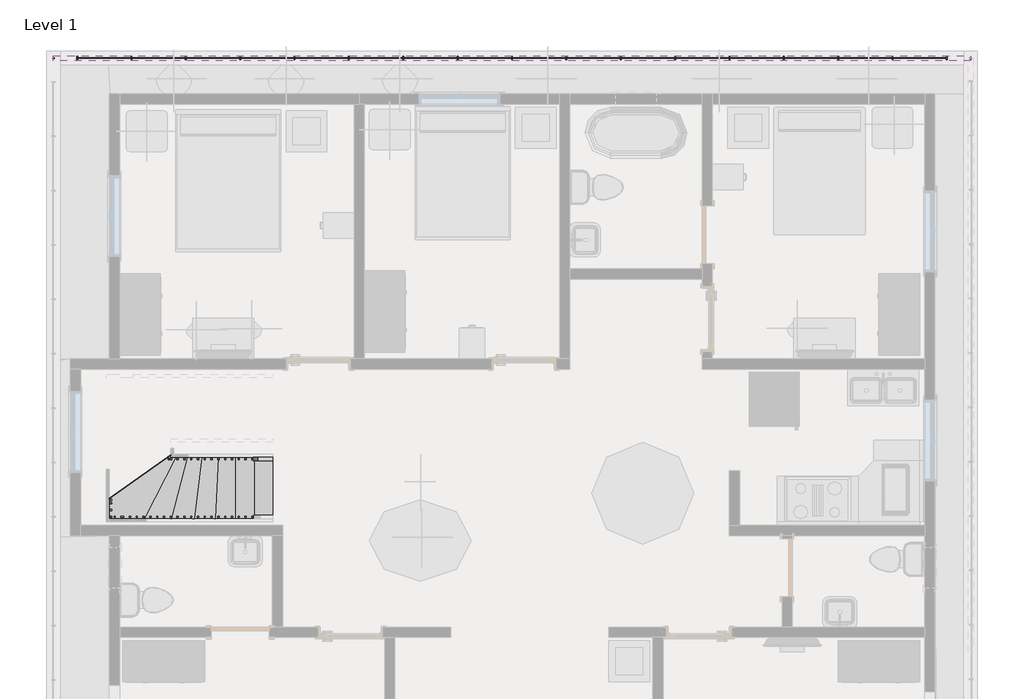
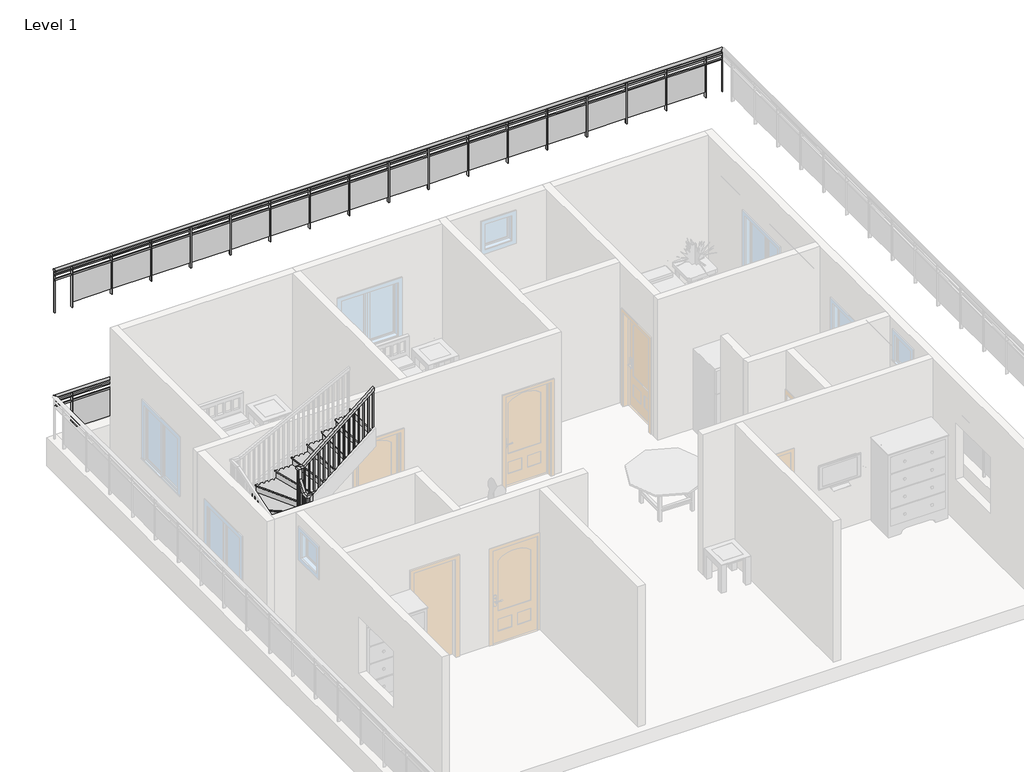
# One storey, part 3 of 5: 3 railings, 1 stair flight.
"""IFC4 building model written with IfcOpenShell, lengths in millimetres."""

from ifc_helpers import new_model, si_unit, point, frame, origin, place, context, project, spatial, polyline, ellipse_curve, trimmed, outline, extrude, faceted_brep, transform, mapped, element, save
from ifc_brep_helpers import plane_surface, extruded_surface, advanced_brep
from components import stair_flight_b82eb699

model = new_model("IFC4")

# Units and contexts
model_context = context("Model", 3, world=origin())
ifc_project = project(units=[si_unit("LENGTHUNIT", "METRE", prefix="MILLI")], contexts=[model_context])

# Site, building, storey
site = spatial("IfcSite", under=ifc_project)
building = spatial("IfcBuilding", under=site)
storey = spatial("IfcBuildingStorey", under=building, Name="Level 1", Elevation=0.0)

# Railings
placement = place(None, origin())
element("IfcRailing", 1, ObjectType="Glass Panel - Bottom Fill", at=placement, inside=storey, context=model_context, shape_type="SolidModel", body=[
    advanced_brep(
    [(-11479.0434666, 14380.2716937, 4267.2), (-11479.0434666, 14304.0716937, 4267.2), (2236.9565334, 14380.2716937, 4267.2), (2236.9565334, 14304.0716937, 4267.2)],
    [
        (0, 1, ellipse_curve(frame((-11479.0434666, 14342.1716937, 4267.2), z_axis=(-1.0, 0.0, 0.0), x_axis=(0.0, -1.0, 0.0)), 38.1, 28.575)),
        (1, 0, ellipse_curve(frame((-11479.0434666, 14342.1716937, 4267.2), z_axis=(-1.0, 0.0, 0.0), x_axis=(0.0, -1.0, 0.0)), 38.1, 28.575)),
        (2, 3, ellipse_curve(frame((2236.9565334, 14342.1716937, 4267.2), z_axis=(1.0, 0.0, 0.0), x_axis=(0.0, -1.0, 0.0)), 38.1, 28.575)),
        (3, 2, ellipse_curve(frame((2236.9565334, 14342.1716937, 4267.2), z_axis=(1.0, 0.0, 0.0), x_axis=(0.0, -1.0, 0.0)), 38.1, 28.575)),
        (0, 2),
        (3, 1),
    ],
    [
        plane_surface(frame((-11479.0434666, 14342.1716937, 4267.2), z_axis=(-1.0, 0.0, 0.0), x_axis=(0.0, 1.0, 0.0))),
        plane_surface(frame((2236.9565334, 14342.1716937, 4267.2), z_axis=(1.0, 0.0, 0.0), x_axis=(0.0, 1.0, 0.0))),
        extruded_surface(trimmed(ellipse_curve(frame((2236.9565334, 14342.1716937, 4267.2), z_axis=(-1.0, 0.0, 0.0), x_axis=(0.0, -1.0, 0.0)), 38.1, 28.575), [point((2236.9565334, 14380.2716937, 4267.2))], [point((2236.9565334, 14304.0716937, 4267.2))], True, "CARTESIAN"), (-13716.0, 0.0, 0.0), 13716.0),
        extruded_surface(trimmed(ellipse_curve(frame((2236.9565334, 14342.1716937, 4267.2), z_axis=(-1.0, 0.0, 0.0), x_axis=(0.0, -1.0, 0.0)), 38.1, 28.575), [point((2236.9565334, 14304.0716937, 4267.2))], [point((2236.9565334, 14380.2716937, 4267.2))], True, "CARTESIAN"), (-13716.0, 0.0, 0.0), 13716.0),
    ],
    [
        (0, [[1, 2]]),
        (1, [[3, 4]]),
        (2, [[-1, 5, -4, 6]]),
        (3, [[-2, -6, -3, -5]]),
    ],
),
    extrude(outline(polyline([(-11479.0434666, 14329.4716937), (-11479.0434666, 14354.8716937), (2236.9565334, 14354.8716937), (2236.9565334, 14329.4716937), (-11479.0434666, 14329.4716937)])), frame((0.0, 0.0, 4152.9), z_axis=(0.0, 0.0, 1.0), x_axis=(1.0, 0.0, 0.0)), (0.0, 0.0, 1.0), 25.4),
    extrude(outline(polyline([(-11479.0434666, 14329.4716937), (-11479.0434666, 14354.8716937), (2236.9565334, 14354.8716937), (2236.9565334, 14329.4716937), (-11479.0434666, 14329.4716937)])), frame((0.0, 0.0, 4051.3), z_axis=(0.0, 0.0, 1.0), x_axis=(1.0, 0.0, 0.0)), (0.0, 0.0, 1.0), 25.4),
    extrude(outline(polyline([(1875.0065334, 14316.7716937), (1875.0065334, 14367.5716937), (1887.7065334, 14367.5716937), (1887.7065334, 14316.7716937), (1875.0065334, 14316.7716937)])), frame((0.0, 0.0, 3352.8), z_axis=(0.0, 0.0, 1.0), x_axis=(1.0, 0.0, 0.0)), (0.0, 0.0, 1.0), 885.6788223),
    extrude(outline(polyline([(1068.5565334, 14348.7068507), (1881.3565334, 14348.7068507), (1881.3565334, 14342.3568507), (1068.5565334, 14342.3568507), (1068.5565334, 14348.7068507)])), frame((0.0, 0.0, 3454.4), z_axis=(0.0, 0.0, 1.0), x_axis=(1.0, 0.0, 0.0)), (0.0, 0.0, 1.0), 596.9),
    extrude(outline(polyline([(1062.2065334, 14316.7716937), (1062.2065334, 14367.5716937), (1074.9065334, 14367.5716937), (1074.9065334, 14316.7716937), (1062.2065334, 14316.7716937)])), frame((0.0, 0.0, 3352.8), z_axis=(0.0, 0.0, 1.0), x_axis=(1.0, 0.0, 0.0)), (0.0, 0.0, 1.0), 885.6788223),
    extrude(outline(polyline([(255.7565334, 14348.7068507), (1068.5565334, 14348.7068507), (1068.5565334, 14342.3568507), (255.7565334, 14342.3568507), (255.7565334, 14348.7068507)])), frame((0.0, 0.0, 3454.4), z_axis=(0.0, 0.0, 1.0), x_axis=(1.0, 0.0, 0.0)), (0.0, 0.0, 1.0), 596.9),
    extrude(outline(polyline([(249.4065334, 14316.7716937), (249.4065334, 14367.5716937), (262.1065334, 14367.5716937), (262.1065334, 14316.7716937), (249.4065334, 14316.7716937)])), frame((0.0, 0.0, 3352.8), z_axis=(0.0, 0.0, 1.0), x_axis=(1.0, 0.0, 0.0)), (0.0, 0.0, 1.0), 885.6788223),
    extrude(outline(polyline([(-557.0434666, 14348.7068507), (255.7565334, 14348.7068507), (255.7565334, 14342.3568507), (-557.0434666, 14342.3568507), (-557.0434666, 14348.7068507)])), frame((0.0, 0.0, 3454.4), z_axis=(0.0, 0.0, 1.0), x_axis=(1.0, 0.0, 0.0)), (0.0, 0.0, 1.0), 596.9),
    extrude(outline(polyline([(-563.3934666, 14316.7716937), (-563.3934666, 14367.5716937), (-550.6934666, 14367.5716937), (-550.6934666, 14316.7716937), (-563.3934666, 14316.7716937)])), frame((0.0, 0.0, 3352.8), z_axis=(0.0, 0.0, 1.0), x_axis=(1.0, 0.0, 0.0)), (0.0, 0.0, 1.0), 885.6788223),
    extrude(outline(polyline([(-1369.8434666, 14348.7068507), (-557.0434666, 14348.7068507), (-557.0434666, 14342.3568507), (-1369.8434666, 14342.3568507), (-1369.8434666, 14348.7068507)])), frame((0.0, 0.0, 3454.4), z_axis=(0.0, 0.0, 1.0), x_axis=(1.0, 0.0, 0.0)), (0.0, 0.0, 1.0), 596.9),
    extrude(outline(polyline([(-1376.1934666, 14316.7716937), (-1376.1934666, 14367.5716937), (-1363.4934666, 14367.5716937), (-1363.4934666, 14316.7716937), (-1376.1934666, 14316.7716937)])), frame((0.0, 0.0, 3352.8), z_axis=(0.0, 0.0, 1.0), x_axis=(1.0, 0.0, 0.0)), (0.0, 0.0, 1.0), 885.6788223),
    extrude(outline(polyline([(-2182.6434666, 14348.7068507), (-1369.8434666, 14348.7068507), (-1369.8434666, 14342.3568507), (-2182.6434666, 14342.3568507), (-2182.6434666, 14348.7068507)])), frame((0.0, 0.0, 3454.4), z_axis=(0.0, 0.0, 1.0), x_axis=(1.0, 0.0, 0.0)), (0.0, 0.0, 1.0), 596.9),
    extrude(outline(polyline([(-2188.9934666, 14316.7716937), (-2188.9934666, 14367.5716937), (-2176.2934666, 14367.5716937), (-2176.2934666, 14316.7716937), (-2188.9934666, 14316.7716937)])), frame((0.0, 0.0, 3352.8), z_axis=(0.0, 0.0, 1.0), x_axis=(1.0, 0.0, 0.0)), (0.0, 0.0, 1.0), 885.6788223),
    extrude(outline(polyline([(-2995.4434666, 14348.7068507), (-2182.6434666, 14348.7068507), (-2182.6434666, 14342.3568507), (-2995.4434666, 14342.3568507), (-2995.4434666, 14348.7068507)])), frame((0.0, 0.0, 3454.4), z_axis=(0.0, 0.0, 1.0), x_axis=(1.0, 0.0, 0.0)), (0.0, 0.0, 1.0), 596.9),
    extrude(outline(polyline([(-3001.7934666, 14316.7716937), (-3001.7934666, 14367.5716937), (-2989.0934666, 14367.5716937), (-2989.0934666, 14316.7716937), (-3001.7934666, 14316.7716937)])), frame((0.0, 0.0, 3352.8), z_axis=(0.0, 0.0, 1.0), x_axis=(1.0, 0.0, 0.0)), (0.0, 0.0, 1.0), 885.6788223),
    extrude(outline(polyline([(-3808.2434666, 14348.7068507), (-2995.4434666, 14348.7068507), (-2995.4434666, 14342.3568507), (-3808.2434666, 14342.3568507), (-3808.2434666, 14348.7068507)])), frame((0.0, 0.0, 3454.4), z_axis=(0.0, 0.0, 1.0), x_axis=(1.0, 0.0, 0.0)), (0.0, 0.0, 1.0), 596.9),
    extrude(outline(polyline([(-3814.5934666, 14316.7716937), (-3814.5934666, 14367.5716937), (-3801.8934666, 14367.5716937), (-3801.8934666, 14316.7716937), (-3814.5934666, 14316.7716937)])), frame((0.0, 0.0, 3352.8), z_axis=(0.0, 0.0, 1.0), x_axis=(1.0, 0.0, 0.0)), (0.0, 0.0, 1.0), 885.6788223),
    extrude(outline(polyline([(-4621.0434666, 14348.7068507), (-3808.2434666, 14348.7068507), (-3808.2434666, 14342.3568507), (-4621.0434666, 14342.3568507), (-4621.0434666, 14348.7068507)])), frame((0.0, 0.0, 3454.4), z_axis=(0.0, 0.0, 1.0), x_axis=(1.0, 0.0, 0.0)), (0.0, 0.0, 1.0), 596.9),
    extrude(outline(polyline([(-4627.3934666, 14316.7716937), (-4627.3934666, 14367.5716937), (-4614.6934666, 14367.5716937), (-4614.6934666, 14316.7716937), (-4627.3934666, 14316.7716937)])), frame((0.0, 0.0, 3352.8), z_axis=(0.0, 0.0, 1.0), x_axis=(1.0, 0.0, 0.0)), (0.0, 0.0, 1.0), 885.6788223),
    extrude(outline(polyline([(-5433.8434666, 14348.7068507), (-4621.0434666, 14348.7068507), (-4621.0434666, 14342.3568507), (-5433.8434666, 14342.3568507), (-5433.8434666, 14348.7068507)])), frame((0.0, 0.0, 3454.4), z_axis=(0.0, 0.0, 1.0), x_axis=(1.0, 0.0, 0.0)), (0.0, 0.0, 1.0), 596.9),
    extrude(outline(polyline([(-5440.1934666, 14316.7716937), (-5440.1934666, 14367.5716937), (-5427.4934666, 14367.5716937), (-5427.4934666, 14316.7716937), (-5440.1934666, 14316.7716937)])), frame((0.0, 0.0, 3352.8), z_axis=(0.0, 0.0, 1.0), x_axis=(1.0, 0.0, 0.0)), (0.0, 0.0, 1.0), 885.6788223),
    extrude(outline(polyline([(-6246.6434666, 14348.7068507), (-5433.8434666, 14348.7068507), (-5433.8434666, 14342.3568507), (-6246.6434666, 14342.3568507), (-6246.6434666, 14348.7068507)])), frame((0.0, 0.0, 3454.4), z_axis=(0.0, 0.0, 1.0), x_axis=(1.0, 0.0, 0.0)), (0.0, 0.0, 1.0), 596.9),
    extrude(outline(polyline([(-6252.9934666, 14316.7716937), (-6252.9934666, 14367.5716937), (-6240.2934666, 14367.5716937), (-6240.2934666, 14316.7716937), (-6252.9934666, 14316.7716937)])), frame((0.0, 0.0, 3352.8), z_axis=(0.0, 0.0, 1.0), x_axis=(1.0, 0.0, 0.0)), (0.0, 0.0, 1.0), 885.6788223),
    extrude(outline(polyline([(-7059.4434666, 14348.7068507), (-6246.6434666, 14348.7068507), (-6246.6434666, 14342.3568507), (-7059.4434666, 14342.3568507), (-7059.4434666, 14348.7068507)])), frame((0.0, 0.0, 3454.4), z_axis=(0.0, 0.0, 1.0), x_axis=(1.0, 0.0, 0.0)), (0.0, 0.0, 1.0), 596.9),
    extrude(outline(polyline([(-7065.7934666, 14316.7716937), (-7065.7934666, 14367.5716937), (-7053.0934666, 14367.5716937), (-7053.0934666, 14316.7716937), (-7065.7934666, 14316.7716937)])), frame((0.0, 0.0, 3352.8), z_axis=(0.0, 0.0, 1.0), x_axis=(1.0, 0.0, 0.0)), (0.0, 0.0, 1.0), 885.6788223),
    extrude(outline(polyline([(-7872.2434666, 14348.7068507), (-7059.4434666, 14348.7068507), (-7059.4434666, 14342.3568507), (-7872.2434666, 14342.3568507), (-7872.2434666, 14348.7068507)])), frame((0.0, 0.0, 3454.4), z_axis=(0.0, 0.0, 1.0), x_axis=(1.0, 0.0, 0.0)), (0.0, 0.0, 1.0), 596.9),
    extrude(outline(polyline([(-7878.5934666, 14316.7716937), (-7878.5934666, 14367.5716937), (-7865.8934666, 14367.5716937), (-7865.8934666, 14316.7716937), (-7878.5934666, 14316.7716937)])), frame((0.0, 0.0, 3352.8), z_axis=(0.0, 0.0, 1.0), x_axis=(1.0, 0.0, 0.0)), (0.0, 0.0, 1.0), 885.6788223),
    extrude(outline(polyline([(-8685.0434666, 14348.7068507), (-7872.2434666, 14348.7068507), (-7872.2434666, 14342.3568507), (-8685.0434666, 14342.3568507), (-8685.0434666, 14348.7068507)])), frame((0.0, 0.0, 3454.4), z_axis=(0.0, 0.0, 1.0), x_axis=(1.0, 0.0, 0.0)), (0.0, 0.0, 1.0), 596.9),
    extrude(outline(polyline([(-8691.3934666, 14316.7716937), (-8691.3934666, 14367.5716937), (-8678.6934666, 14367.5716937), (-8678.6934666, 14316.7716937), (-8691.3934666, 14316.7716937)])), frame((0.0, 0.0, 3352.8), z_axis=(0.0, 0.0, 1.0), x_axis=(1.0, 0.0, 0.0)), (0.0, 0.0, 1.0), 885.6788223),
    extrude(outline(polyline([(-9497.8434666, 14348.7068507), (-8685.0434666, 14348.7068507), (-8685.0434666, 14342.3568507), (-9497.8434666, 14342.3568507), (-9497.8434666, 14348.7068507)])), frame((0.0, 0.0, 3454.4), z_axis=(0.0, 0.0, 1.0), x_axis=(1.0, 0.0, 0.0)), (0.0, 0.0, 1.0), 596.9),
    extrude(outline(polyline([(-9504.1934666, 14316.7716937), (-9504.1934666, 14367.5716937), (-9491.4934666, 14367.5716937), (-9491.4934666, 14316.7716937), (-9504.1934666, 14316.7716937)])), frame((0.0, 0.0, 3352.8), z_axis=(0.0, 0.0, 1.0), x_axis=(1.0, 0.0, 0.0)), (0.0, 0.0, 1.0), 885.6788223),
    extrude(outline(polyline([(-10310.6434666, 14348.7068507), (-9497.8434666, 14348.7068507), (-9497.8434666, 14342.3568507), (-10310.6434666, 14342.3568507), (-10310.6434666, 14348.7068507)])), frame((0.0, 0.0, 3454.4), z_axis=(0.0, 0.0, 1.0), x_axis=(1.0, 0.0, 0.0)), (0.0, 0.0, 1.0), 596.9),
    extrude(outline(polyline([(-10316.9934666, 14316.7716937), (-10316.9934666, 14367.5716937), (-10304.2934666, 14367.5716937), (-10304.2934666, 14316.7716937), (-10316.9934666, 14316.7716937)])), frame((0.0, 0.0, 3352.8), z_axis=(0.0, 0.0, 1.0), x_axis=(1.0, 0.0, 0.0)), (0.0, 0.0, 1.0), 885.6788223),
    extrude(outline(polyline([(-11123.4434666, 14348.7068507), (-10310.6434666, 14348.7068507), (-10310.6434666, 14342.3568507), (-11123.4434666, 14342.3568507), (-11123.4434666, 14348.7068507)])), frame((0.0, 0.0, 3454.4), z_axis=(0.0, 0.0, 1.0), x_axis=(1.0, 0.0, 0.0)), (0.0, 0.0, 1.0), 596.9),
    extrude(outline(polyline([(-11129.7934666, 14316.7716937), (-11129.7934666, 14367.5716937), (-11117.0934666, 14367.5716937), (-11117.0934666, 14316.7716937), (-11129.7934666, 14316.7716937)])), frame((0.0, 0.0, 3352.8), z_axis=(0.0, 0.0, 1.0), x_axis=(1.0, 0.0, 0.0)), (0.0, 0.0, 1.0), 885.6788223),
    extrude(outline(polyline([(2224.2565334, 14332.6466937), (2224.2565334, 14351.6966937), (2243.3065334, 14351.6966937), (2243.3065334, 14332.6466937), (2224.2565334, 14332.6466937)])), frame((0.0, 0.0, 3352.8), z_axis=(0.0, 0.0, 1.0), x_axis=(1.0, 0.0, 0.0)), (0.0, 0.0, 1.0), 885.6788223),
    extrude(outline(polyline([(-11485.3934666, 14332.6466937), (-11485.3934666, 14351.6966937), (-11466.3434666, 14351.6966937), (-11466.3434666, 14332.6466937), (-11485.3934666, 14332.6466937)])), frame((0.0, 0.0, 3352.8), z_axis=(0.0, 0.0, 1.0), x_axis=(1.0, 0.0, 0.0)), (0.0, 0.0, 1.0), 885.6788223),
])
element("IfcRailing", 2, ObjectType="Glass Panel - Bottom Fill", at=placement, inside=storey, context=model_context, shape_type="SolidModel", body=[
    advanced_brep(
    [(-11479.0434666, 14380.2716937, 1524.0), (-11479.0434666, 14304.0716937, 1524.0), (2236.9565334, 14380.2716937, 1524.0), (2236.9565334, 14304.0716937, 1524.0)],
    [
        (0, 1, ellipse_curve(frame((-11479.0434666, 14342.1716937, 1524.0), z_axis=(-1.0, 0.0, 0.0), x_axis=(0.0, -1.0, 0.0)), 38.1, 28.575)),
        (1, 0, ellipse_curve(frame((-11479.0434666, 14342.1716937, 1524.0), z_axis=(-1.0, 0.0, 0.0), x_axis=(0.0, -1.0, 0.0)), 38.1, 28.575)),
        (2, 3, ellipse_curve(frame((2236.9565334, 14342.1716937, 1524.0), z_axis=(1.0, 0.0, 0.0), x_axis=(0.0, -1.0, 0.0)), 38.1, 28.575)),
        (3, 2, ellipse_curve(frame((2236.9565334, 14342.1716937, 1524.0), z_axis=(1.0, 0.0, 0.0), x_axis=(0.0, -1.0, 0.0)), 38.1, 28.575)),
        (0, 2),
        (3, 1),
    ],
    [
        plane_surface(frame((-11479.0434666, 14342.1716937, 1524.0), z_axis=(-1.0, 0.0, 0.0), x_axis=(0.0, 1.0, 0.0))),
        plane_surface(frame((2236.9565334, 14342.1716937, 1524.0), z_axis=(1.0, 0.0, 0.0), x_axis=(0.0, 1.0, 0.0))),
        extruded_surface(trimmed(ellipse_curve(frame((2236.9565334, 14342.1716937, 1524.0), z_axis=(-1.0, 0.0, 0.0), x_axis=(0.0, -1.0, 0.0)), 38.1, 28.575), [point((2236.9565334, 14380.2716937, 1524.0))], [point((2236.9565334, 14304.0716937, 1524.0))], True, "CARTESIAN"), (-13716.0, 0.0, 0.0), 13716.0),
        extruded_surface(trimmed(ellipse_curve(frame((2236.9565334, 14342.1716937, 1524.0), z_axis=(-1.0, 0.0, 0.0), x_axis=(0.0, -1.0, 0.0)), 38.1, 28.575), [point((2236.9565334, 14304.0716937, 1524.0))], [point((2236.9565334, 14380.2716937, 1524.0))], True, "CARTESIAN"), (-13716.0, 0.0, 0.0), 13716.0),
    ],
    [
        (0, [[1, 2]]),
        (1, [[3, 4]]),
        (2, [[-1, 5, -4, 6]]),
        (3, [[-2, -6, -3, -5]]),
    ],
),
    extrude(outline(polyline([(-11479.0434666, 14329.4716937), (-11479.0434666, 14354.8716937), (2236.9565334, 14354.8716937), (2236.9565334, 14329.4716937), (-11479.0434666, 14329.4716937)])), frame((0.0, 0.0, 1409.7), z_axis=(0.0, 0.0, 1.0), x_axis=(1.0, 0.0, 0.0)), (0.0, 0.0, 1.0), 25.4),
    extrude(outline(polyline([(-11479.0434666, 14329.4716937), (-11479.0434666, 14354.8716937), (2236.9565334, 14354.8716937), (2236.9565334, 14329.4716937), (-11479.0434666, 14329.4716937)])), frame((0.0, 0.0, 1308.1), z_axis=(0.0, 0.0, 1.0), x_axis=(1.0, 0.0, 0.0)), (0.0, 0.0, 1.0), 25.4),
    extrude(outline(polyline([(1875.0065334, 14316.7716937), (1875.0065334, 14367.5716937), (1887.7065334, 14367.5716937), (1887.7065334, 14316.7716937), (1875.0065334, 14316.7716937)])), frame((0.0, 0.0, 609.6), z_axis=(0.0, 0.0, 1.0), x_axis=(1.0, 0.0, 0.0)), (0.0, 0.0, 1.0), 885.6788223),
    extrude(outline(polyline([(1068.5565334, 14348.7068507), (1881.3565334, 14348.7068507), (1881.3565334, 14342.3568507), (1068.5565334, 14342.3568507), (1068.5565334, 14348.7068507)])), frame((0.0, 0.0, 711.2), z_axis=(0.0, 0.0, 1.0), x_axis=(1.0, 0.0, 0.0)), (0.0, 0.0, 1.0), 596.9),
    extrude(outline(polyline([(1062.2065334, 14316.7716937), (1062.2065334, 14367.5716937), (1074.9065334, 14367.5716937), (1074.9065334, 14316.7716937), (1062.2065334, 14316.7716937)])), frame((0.0, 0.0, 609.6), z_axis=(0.0, 0.0, 1.0), x_axis=(1.0, 0.0, 0.0)), (0.0, 0.0, 1.0), 885.6788223),
    extrude(outline(polyline([(255.7565334, 14348.7068507), (1068.5565334, 14348.7068507), (1068.5565334, 14342.3568507), (255.7565334, 14342.3568507), (255.7565334, 14348.7068507)])), frame((0.0, 0.0, 711.2), z_axis=(0.0, 0.0, 1.0), x_axis=(1.0, 0.0, 0.0)), (0.0, 0.0, 1.0), 596.9),
    extrude(outline(polyline([(249.4065334, 14316.7716937), (249.4065334, 14367.5716937), (262.1065334, 14367.5716937), (262.1065334, 14316.7716937), (249.4065334, 14316.7716937)])), frame((0.0, 0.0, 609.6), z_axis=(0.0, 0.0, 1.0), x_axis=(1.0, 0.0, 0.0)), (0.0, 0.0, 1.0), 885.6788223),
    extrude(outline(polyline([(-557.0434666, 14348.7068507), (255.7565334, 14348.7068507), (255.7565334, 14342.3568507), (-557.0434666, 14342.3568507), (-557.0434666, 14348.7068507)])), frame((0.0, 0.0, 711.2), z_axis=(0.0, 0.0, 1.0), x_axis=(1.0, 0.0, 0.0)), (0.0, 0.0, 1.0), 596.9),
    extrude(outline(polyline([(-563.3934666, 14316.7716937), (-563.3934666, 14367.5716937), (-550.6934666, 14367.5716937), (-550.6934666, 14316.7716937), (-563.3934666, 14316.7716937)])), frame((0.0, 0.0, 609.6), z_axis=(0.0, 0.0, 1.0), x_axis=(1.0, 0.0, 0.0)), (0.0, 0.0, 1.0), 885.6788223),
    extrude(outline(polyline([(-1369.8434666, 14348.7068507), (-557.0434666, 14348.7068507), (-557.0434666, 14342.3568507), (-1369.8434666, 14342.3568507), (-1369.8434666, 14348.7068507)])), frame((0.0, 0.0, 711.2), z_axis=(0.0, 0.0, 1.0), x_axis=(1.0, 0.0, 0.0)), (0.0, 0.0, 1.0), 596.9),
    extrude(outline(polyline([(-1376.1934666, 14316.7716937), (-1376.1934666, 14367.5716937), (-1363.4934666, 14367.5716937), (-1363.4934666, 14316.7716937), (-1376.1934666, 14316.7716937)])), frame((0.0, 0.0, 609.6), z_axis=(0.0, 0.0, 1.0), x_axis=(1.0, 0.0, 0.0)), (0.0, 0.0, 1.0), 885.6788223),
    extrude(outline(polyline([(-2182.6434666, 14348.7068507), (-1369.8434666, 14348.7068507), (-1369.8434666, 14342.3568507), (-2182.6434666, 14342.3568507), (-2182.6434666, 14348.7068507)])), frame((0.0, 0.0, 711.2), z_axis=(0.0, 0.0, 1.0), x_axis=(1.0, 0.0, 0.0)), (0.0, 0.0, 1.0), 596.9),
    extrude(outline(polyline([(-2188.9934666, 14316.7716937), (-2188.9934666, 14367.5716937), (-2176.2934666, 14367.5716937), (-2176.2934666, 14316.7716937), (-2188.9934666, 14316.7716937)])), frame((0.0, 0.0, 609.6), z_axis=(0.0, 0.0, 1.0), x_axis=(1.0, 0.0, 0.0)), (0.0, 0.0, 1.0), 885.6788223),
    extrude(outline(polyline([(-2995.4434666, 14348.7068507), (-2182.6434666, 14348.7068507), (-2182.6434666, 14342.3568507), (-2995.4434666, 14342.3568507), (-2995.4434666, 14348.7068507)])), frame((0.0, 0.0, 711.2), z_axis=(0.0, 0.0, 1.0), x_axis=(1.0, 0.0, 0.0)), (0.0, 0.0, 1.0), 596.9),
    extrude(outline(polyline([(-3001.7934666, 14316.7716937), (-3001.7934666, 14367.5716937), (-2989.0934666, 14367.5716937), (-2989.0934666, 14316.7716937), (-3001.7934666, 14316.7716937)])), frame((0.0, 0.0, 609.6), z_axis=(0.0, 0.0, 1.0), x_axis=(1.0, 0.0, 0.0)), (0.0, 0.0, 1.0), 885.6788223),
    extrude(outline(polyline([(-3808.2434666, 14348.7068507), (-2995.4434666, 14348.7068507), (-2995.4434666, 14342.3568507), (-3808.2434666, 14342.3568507), (-3808.2434666, 14348.7068507)])), frame((0.0, 0.0, 711.2), z_axis=(0.0, 0.0, 1.0), x_axis=(1.0, 0.0, 0.0)), (0.0, 0.0, 1.0), 596.9),
    extrude(outline(polyline([(-3814.5934666, 14316.7716937), (-3814.5934666, 14367.5716937), (-3801.8934666, 14367.5716937), (-3801.8934666, 14316.7716937), (-3814.5934666, 14316.7716937)])), frame((0.0, 0.0, 609.6), z_axis=(0.0, 0.0, 1.0), x_axis=(1.0, 0.0, 0.0)), (0.0, 0.0, 1.0), 885.6788223),
    extrude(outline(polyline([(-4621.0434666, 14348.7068507), (-3808.2434666, 14348.7068507), (-3808.2434666, 14342.3568507), (-4621.0434666, 14342.3568507), (-4621.0434666, 14348.7068507)])), frame((0.0, 0.0, 711.2), z_axis=(0.0, 0.0, 1.0), x_axis=(1.0, 0.0, 0.0)), (0.0, 0.0, 1.0), 596.9),
    extrude(outline(polyline([(-4627.3934666, 14316.7716937), (-4627.3934666, 14367.5716937), (-4614.6934666, 14367.5716937), (-4614.6934666, 14316.7716937), (-4627.3934666, 14316.7716937)])), frame((0.0, 0.0, 609.6), z_axis=(0.0, 0.0, 1.0), x_axis=(1.0, 0.0, 0.0)), (0.0, 0.0, 1.0), 885.6788223),
    extrude(outline(polyline([(-5433.8434666, 14348.7068507), (-4621.0434666, 14348.7068507), (-4621.0434666, 14342.3568507), (-5433.8434666, 14342.3568507), (-5433.8434666, 14348.7068507)])), frame((0.0, 0.0, 711.2), z_axis=(0.0, 0.0, 1.0), x_axis=(1.0, 0.0, 0.0)), (0.0, 0.0, 1.0), 596.9),
    extrude(outline(polyline([(-5440.1934666, 14316.7716937), (-5440.1934666, 14367.5716937), (-5427.4934666, 14367.5716937), (-5427.4934666, 14316.7716937), (-5440.1934666, 14316.7716937)])), frame((0.0, 0.0, 609.6), z_axis=(0.0, 0.0, 1.0), x_axis=(1.0, 0.0, 0.0)), (0.0, 0.0, 1.0), 885.6788223),
    extrude(outline(polyline([(-6246.6434666, 14348.7068507), (-5433.8434666, 14348.7068507), (-5433.8434666, 14342.3568507), (-6246.6434666, 14342.3568507), (-6246.6434666, 14348.7068507)])), frame((0.0, 0.0, 711.2), z_axis=(0.0, 0.0, 1.0), x_axis=(1.0, 0.0, 0.0)), (0.0, 0.0, 1.0), 596.9),
    extrude(outline(polyline([(-6252.9934666, 14316.7716937), (-6252.9934666, 14367.5716937), (-6240.2934666, 14367.5716937), (-6240.2934666, 14316.7716937), (-6252.9934666, 14316.7716937)])), frame((0.0, 0.0, 609.6), z_axis=(0.0, 0.0, 1.0), x_axis=(1.0, 0.0, 0.0)), (0.0, 0.0, 1.0), 885.6788223),
    extrude(outline(polyline([(-7059.4434666, 14348.7068507), (-6246.6434666, 14348.7068507), (-6246.6434666, 14342.3568507), (-7059.4434666, 14342.3568507), (-7059.4434666, 14348.7068507)])), frame((0.0, 0.0, 711.2), z_axis=(0.0, 0.0, 1.0), x_axis=(1.0, 0.0, 0.0)), (0.0, 0.0, 1.0), 596.9),
    extrude(outline(polyline([(-7065.7934666, 14316.7716937), (-7065.7934666, 14367.5716937), (-7053.0934666, 14367.5716937), (-7053.0934666, 14316.7716937), (-7065.7934666, 14316.7716937)])), frame((0.0, 0.0, 609.6), z_axis=(0.0, 0.0, 1.0), x_axis=(1.0, 0.0, 0.0)), (0.0, 0.0, 1.0), 885.6788223),
    extrude(outline(polyline([(-7872.2434666, 14348.7068507), (-7059.4434666, 14348.7068507), (-7059.4434666, 14342.3568507), (-7872.2434666, 14342.3568507), (-7872.2434666, 14348.7068507)])), frame((0.0, 0.0, 711.2), z_axis=(0.0, 0.0, 1.0), x_axis=(1.0, 0.0, 0.0)), (0.0, 0.0, 1.0), 596.9),
    extrude(outline(polyline([(-7878.5934666, 14316.7716937), (-7878.5934666, 14367.5716937), (-7865.8934666, 14367.5716937), (-7865.8934666, 14316.7716937), (-7878.5934666, 14316.7716937)])), frame((0.0, 0.0, 609.6), z_axis=(0.0, 0.0, 1.0), x_axis=(1.0, 0.0, 0.0)), (0.0, 0.0, 1.0), 885.6788223),
    extrude(outline(polyline([(-8685.0434666, 14348.7068507), (-7872.2434666, 14348.7068507), (-7872.2434666, 14342.3568507), (-8685.0434666, 14342.3568507), (-8685.0434666, 14348.7068507)])), frame((0.0, 0.0, 711.2), z_axis=(0.0, 0.0, 1.0), x_axis=(1.0, 0.0, 0.0)), (0.0, 0.0, 1.0), 596.9),
    extrude(outline(polyline([(-8691.3934666, 14316.7716937), (-8691.3934666, 14367.5716937), (-8678.6934666, 14367.5716937), (-8678.6934666, 14316.7716937), (-8691.3934666, 14316.7716937)])), frame((0.0, 0.0, 609.6), z_axis=(0.0, 0.0, 1.0), x_axis=(1.0, 0.0, 0.0)), (0.0, 0.0, 1.0), 885.6788223),
    extrude(outline(polyline([(-9497.8434666, 14348.7068507), (-8685.0434666, 14348.7068507), (-8685.0434666, 14342.3568507), (-9497.8434666, 14342.3568507), (-9497.8434666, 14348.7068507)])), frame((0.0, 0.0, 711.2), z_axis=(0.0, 0.0, 1.0), x_axis=(1.0, 0.0, 0.0)), (0.0, 0.0, 1.0), 596.9),
    extrude(outline(polyline([(-9504.1934666, 14316.7716937), (-9504.1934666, 14367.5716937), (-9491.4934666, 14367.5716937), (-9491.4934666, 14316.7716937), (-9504.1934666, 14316.7716937)])), frame((0.0, 0.0, 609.6), z_axis=(0.0, 0.0, 1.0), x_axis=(1.0, 0.0, 0.0)), (0.0, 0.0, 1.0), 885.6788223),
    extrude(outline(polyline([(-10310.6434666, 14348.7068507), (-9497.8434666, 14348.7068507), (-9497.8434666, 14342.3568507), (-10310.6434666, 14342.3568507), (-10310.6434666, 14348.7068507)])), frame((0.0, 0.0, 711.2), z_axis=(0.0, 0.0, 1.0), x_axis=(1.0, 0.0, 0.0)), (0.0, 0.0, 1.0), 596.9),
    extrude(outline(polyline([(-10316.9934666, 14316.7716937), (-10316.9934666, 14367.5716937), (-10304.2934666, 14367.5716937), (-10304.2934666, 14316.7716937), (-10316.9934666, 14316.7716937)])), frame((0.0, 0.0, 609.6), z_axis=(0.0, 0.0, 1.0), x_axis=(1.0, 0.0, 0.0)), (0.0, 0.0, 1.0), 885.6788223),
    extrude(outline(polyline([(-11123.4434666, 14348.7068507), (-10310.6434666, 14348.7068507), (-10310.6434666, 14342.3568507), (-11123.4434666, 14342.3568507), (-11123.4434666, 14348.7068507)])), frame((0.0, 0.0, 711.2), z_axis=(0.0, 0.0, 1.0), x_axis=(1.0, 0.0, 0.0)), (0.0, 0.0, 1.0), 596.9),
    extrude(outline(polyline([(-11129.7934666, 14316.7716937), (-11129.7934666, 14367.5716937), (-11117.0934666, 14367.5716937), (-11117.0934666, 14316.7716937), (-11129.7934666, 14316.7716937)])), frame((0.0, 0.0, 609.6), z_axis=(0.0, 0.0, 1.0), x_axis=(1.0, 0.0, 0.0)), (0.0, 0.0, 1.0), 885.6788223),
    extrude(outline(polyline([(2224.2565334, 14332.6466937), (2224.2565334, 14351.6966937), (2243.3065334, 14351.6966937), (2243.3065334, 14332.6466937), (2224.2565334, 14332.6466937)])), frame((0.0, 0.0, 609.6), z_axis=(0.0, 0.0, 1.0), x_axis=(1.0, 0.0, 0.0)), (0.0, 0.0, 1.0), 885.6788223),
    extrude(outline(polyline([(-11485.3934666, 14332.6466937), (-11485.3934666, 14351.6966937), (-11466.3434666, 14351.6966937), (-11466.3434666, 14332.6466937), (-11485.3934666, 14332.6466937)])), frame((0.0, 0.0, 609.6), z_axis=(0.0, 0.0, 1.0), x_axis=(1.0, 0.0, 0.0)), (0.0, 0.0, 1.0), 885.6788223),
])
element("IfcRailing", 3, ObjectType="Handrail - Rectangular", at=placement, inside=storey, context=model_context, shape_type="SolidModel", body=[
    faceted_brep([(-8198.7117747, 8322.3716937, 1025.2529681), (-8198.7117747, 8322.3716937, 959.7067088), (-8198.7117747, 8373.1716937, 959.7067088), (-8198.7117747, 8373.1716937, 1025.2529681), (-9650.2434666, 8322.3716937, 2208.7848338), (-9701.0434666, 8322.3716937, 2184.659247), (-9701.0434666, 8373.1716937, 2184.659247), (-9650.2434666, 8373.1716937, 2208.7848338), (-9650.2434666, 8322.3716937, 2414.6281882), (-9701.0434666, 8322.3716937, 2363.8281882), (-9701.0434666, 8373.1716937, 2363.8281882), (-9650.2434666, 8373.1716937, 2414.6281882), (-9777.2434666, 8322.3716937, 2414.6281882), (-9777.2434666, 8322.3716937, 2363.8281882), (-9726.4434666, 8373.1716937, 2363.8281882), (-9726.4434666, 8373.1716937, 2414.6281882), (-9777.2434666, 8449.3716937, 2414.6281882), (-9777.2434666, 8478.4930275, 2363.8281882), (-9726.4434666, 8478.4930275, 2363.8281882), (-9726.4434666, 8449.3716937, 2414.6281882), (-9777.2434666, 8576.3716937, 2631.5051451), (-9777.2434666, 8627.1716937, 2617.7256424), (-9726.4434666, 8627.1716937, 2617.7256424), (-9726.4434666, 8576.3716937, 2631.5051451), (-9777.2434666, 8576.3716937, 2837.3484995), (-9777.2434666, 8627.1716937, 2786.5484995), (-9726.4434666, 8627.1716937, 2786.5484995), (-9726.4434666, 8576.3716937, 2837.3484995), (-9777.2434666, 8703.3716937, 2837.3484995), (-9777.2434666, 8703.3716937, 2786.5484995), (-9726.4434666, 8652.5716937, 2786.5484995), (-9726.4434666, 8652.5716937, 2837.3484995), (-9650.2434666, 8703.3716937, 2837.3484995), (-9632.1580535, 8703.3716937, 2786.5484995), (-9632.1580535, 8652.5716937, 2786.5484995), (-9650.2434666, 8652.5716937, 2837.3484995), (-8198.7117747, 8703.3716937, 4020.8803652), (-8198.7117747, 8652.5716937, 4020.8803652), (-8198.7117747, 8652.5716937, 3955.3341059), (-8198.7117747, 8703.3716937, 3955.3341059)], [[[0, 1, 2, 3]], [[1, 0, 4, 5]], [[2, 1, 5, 6]], [[3, 2, 6, 7]], [[0, 3, 7, 4]], [[5, 4, 8, 9]], [[6, 5, 9, 10]], [[7, 6, 10, 11]], [[4, 7, 11, 8]], [[9, 8, 12, 13]], [[10, 9, 13, 14]], [[11, 10, 14, 15]], [[8, 11, 15, 12]], [[13, 12, 16, 17]], [[14, 13, 17, 18]], [[15, 14, 18, 19]], [[12, 15, 19, 16]], [[17, 16, 20, 21]], [[18, 17, 21, 22]], [[19, 18, 22, 23]], [[16, 19, 23, 20]], [[21, 20, 24, 25]], [[22, 21, 25, 26]], [[23, 22, 26, 27]], [[20, 23, 27, 24]], [[25, 24, 28, 29]], [[26, 25, 29, 30]], [[27, 26, 30, 31]], [[24, 27, 31, 28]], [[29, 28, 32, 33]], [[30, 29, 33, 34]], [[31, 30, 34, 35]], [[28, 31, 35, 32]], [[36, 37, 38, 39]], [[33, 32, 36, 39]], [[34, 33, 39, 38]], [[35, 34, 38, 37]], [[32, 35, 37, 36]]]),
    extrude(outline(polyline([(3881.7558784, -8288.9511103), (3866.2231262, -8308.0011103), (2878.6666667, -8308.0011103), (2878.6666667, -8288.9511103), (3881.7558784, -8288.9511103)])), frame((0.0, 8668.4466937, 0.0), z_axis=(0.0, 1.0, 0.0), x_axis=(0.0, 0.0, 1.0)), (0.0, 0.0, 1.0), 19.05),
    extrude(outline(polyline([(3798.9145334, -8390.5511103), (3783.3817813, -8409.6011103), (2878.6666667, -8409.6011103), (2878.6666667, -8390.5511103), (3798.9145334, -8390.5511103)])), frame((0.0, 8668.4466937, 0.0), z_axis=(0.0, 1.0, 0.0), x_axis=(0.0, 0.0, 1.0)), (0.0, 0.0, 1.0), 19.05),
    extrude(outline(polyline([(3716.0731885, -8492.1511103), (3700.5404364, -8511.2011103), (2709.3333333, -8511.2011103), (2709.3333333, -8492.1511103), (3716.0731885, -8492.1511103)])), frame((0.0, 8668.4466937, 0.0), z_axis=(0.0, 1.0, 0.0), x_axis=(0.0, 0.0, 1.0)), (0.0, 0.0, 1.0), 19.05),
    extrude(outline(polyline([(3633.2318436, -8593.7511103), (3617.6990914, -8612.8011103), (2709.3333333, -8612.8011103), (2709.3333333, -8593.7511103), (3633.2318436, -8593.7511103)])), frame((0.0, 8668.4466937, 0.0), z_axis=(0.0, 1.0, 0.0), x_axis=(0.0, 0.0, 1.0)), (0.0, 0.0, 1.0), 19.05),
    extrude(outline(polyline([(3550.3904987, -8695.3511103), (3534.8577465, -8714.4011103), (2709.3333333, -8714.4011103), (2709.3333333, -8695.3511103), (3550.3904987, -8695.3511103)])), frame((0.0, 8668.4466937, 0.0), z_axis=(0.0, 1.0, 0.0), x_axis=(0.0, 0.0, 1.0)), (0.0, 0.0, 1.0), 19.05),
    extrude(outline(polyline([(3467.5491538, -8796.9511103), (3452.0164016, -8816.0011103), (2540.0, -8816.0011103), (2540.0, -8796.9511103), (3467.5491538, -8796.9511103)])), frame((0.0, 8668.4466937, 0.0), z_axis=(0.0, 1.0, 0.0), x_axis=(0.0, 0.0, 1.0)), (0.0, 0.0, 1.0), 19.05),
    extrude(outline(polyline([(3384.7078088, -8898.5511103), (3369.1750567, -8917.6011103), (2540.0, -8917.6011103), (2540.0, -8898.5511103), (3384.7078088, -8898.5511103)])), frame((0.0, 8668.4466937, 0.0), z_axis=(0.0, 1.0, 0.0), x_axis=(0.0, 0.0, 1.0)), (0.0, 0.0, 1.0), 19.05),
    extrude(outline(polyline([(3301.8664639, -9000.1511103), (3286.3337117, -9019.2011103), (2540.0, -9019.2011103), (2540.0, -9000.1511103), (3301.8664639, -9000.1511103)])), frame((0.0, 8668.4466937, 0.0), z_axis=(0.0, 1.0, 0.0), x_axis=(0.0, 0.0, 1.0)), (0.0, 0.0, 1.0), 19.05),
    extrude(outline(polyline([(3219.025119, -9101.7511103), (3203.4923668, -9120.8011103), (2370.6666667, -9120.8011103), (2370.6666667, -9101.7511103), (3219.025119, -9101.7511103)])), frame((0.0, 8668.4466937, 0.0), z_axis=(0.0, 1.0, 0.0), x_axis=(0.0, 0.0, 1.0)), (0.0, 0.0, 1.0), 19.05),
    extrude(outline(polyline([(3136.1837741, -9203.3511103), (3120.6510219, -9222.4011103), (2370.6666667, -9222.4011103), (2370.6666667, -9203.3511103), (3136.1837741, -9203.3511103)])), frame((0.0, 8668.4466937, 0.0), z_axis=(0.0, 1.0, 0.0), x_axis=(0.0, 0.0, 1.0)), (0.0, 0.0, 1.0), 19.05),
    extrude(outline(polyline([(3053.3424291, -9304.9511103), (3037.809677, -9324.0011103), (2201.3333333, -9324.0011103), (2201.3333333, -9304.9511103), (3053.3424291, -9304.9511103)])), frame((0.0, 8668.4466937, 0.0), z_axis=(0.0, 1.0, 0.0), x_axis=(0.0, 0.0, 1.0)), (0.0, 0.0, 1.0), 19.05),
    extrude(outline(polyline([(2970.5010842, -9406.5511103), (2954.9683321, -9425.6011103), (2201.3333333, -9425.6011103), (2201.3333333, -9406.5511103), (2970.5010842, -9406.5511103)])), frame((0.0, 8668.4466937, 0.0), z_axis=(0.0, 1.0, 0.0), x_axis=(0.0, 0.0, 1.0)), (0.0, 0.0, 1.0), 19.05),
    extrude(outline(polyline([(2887.6597393, -9508.1511103), (2872.1269871, -9527.2011103), (2032.0, -9527.2011103), (2032.0, -9508.1511103), (2887.6597393, -9508.1511103)])), frame((0.0, 8668.4466937, 0.0), z_axis=(0.0, 1.0, 0.0), x_axis=(0.0, 0.0, 1.0)), (0.0, 0.0, 1.0), 19.05),
    extrude(outline(polyline([(2804.8183944, -9609.7511103), (2789.2856422, -9628.8011103), (2032.0, -9628.8011103), (2032.0, -9609.7511103), (2804.8183944, -9609.7511103)])), frame((0.0, 8668.4466937, 0.0), z_axis=(0.0, 1.0, 0.0), x_axis=(0.0, 0.0, 1.0)), (0.0, 0.0, 1.0), 19.05),
    extrude(outline(polyline([(8556.2325975, 2496.5834745), (8575.2825975, 2529.115018), (8575.2825975, 1524.0), (8556.2325975, 1524.0), (8556.2325975, 2496.5834745)])), frame((-9761.3684666, 0.0, 0.0), z_axis=(1.0, 0.0, 0.0), x_axis=(0.0, 1.0, 0.0)), (0.0, 0.0, 1.0), 19.05),
    extrude(outline(polyline([(8454.6325975, 2323.0819089), (8473.6825975, 2355.6134525), (8473.6825975, 1524.0), (8454.6325975, 1524.0), (8454.6325975, 2323.0819089)])), frame((-9761.3684666, 0.0, 0.0), z_axis=(1.0, 0.0, 0.0), x_axis=(0.0, 1.0, 0.0)), (0.0, 0.0, 1.0), 19.05),
    extrude(outline(polyline([(2111.7191617, -9611.5867747), (2127.2519138, -9630.6367747), (1016.0, -9630.6367747), (1016.0, -9611.5867747), (2111.7191617, -9611.5867747)])), frame((0.0, 8338.2466937, 0.0), z_axis=(0.0, 1.0, 0.0), x_axis=(0.0, 0.0, 1.0)), (0.0, 0.0, 1.0), 19.05),
    extrude(outline(polyline([(2028.8778167, -9509.9867747), (2044.4105689, -9529.0367747), (1016.0, -9529.0367747), (1016.0, -9509.9867747), (2028.8778167, -9509.9867747)])), frame((0.0, 8338.2466937, 0.0), z_axis=(0.0, 1.0, 0.0), x_axis=(0.0, 0.0, 1.0)), (0.0, 0.0, 1.0), 19.05),
    extrude(outline(polyline([(1946.0364718, -9408.3867747), (1961.569224, -9427.4367747), (846.6666667, -9427.4367747), (846.6666667, -9408.3867747), (1946.0364718, -9408.3867747)])), frame((0.0, 8338.2466937, 0.0), z_axis=(0.0, 1.0, 0.0), x_axis=(0.0, 0.0, 1.0)), (0.0, 0.0, 1.0), 19.05),
    extrude(outline(polyline([(1863.1951269, -9306.7867747), (1878.7278791, -9325.8367747), (846.6666667, -9325.8367747), (846.6666667, -9306.7867747), (1863.1951269, -9306.7867747)])), frame((0.0, 8338.2466937, 0.0), z_axis=(0.0, 1.0, 0.0), x_axis=(0.0, 0.0, 1.0)), (0.0, 0.0, 1.0), 19.05),
    extrude(outline(polyline([(1780.353782, -9205.1867747), (1795.8865341, -9224.2367747), (677.3333333, -9224.2367747), (677.3333333, -9205.1867747), (1780.353782, -9205.1867747)])), frame((0.0, 8338.2466937, 0.0), z_axis=(0.0, 1.0, 0.0), x_axis=(0.0, 0.0, 1.0)), (0.0, 0.0, 1.0), 19.05),
    extrude(outline(polyline([(1697.5124371, -9103.5867747), (1713.0451892, -9122.6367747), (677.3333333, -9122.6367747), (677.3333333, -9103.5867747), (1697.5124371, -9103.5867747)])), frame((0.0, 8338.2466937, 0.0), z_axis=(0.0, 1.0, 0.0), x_axis=(0.0, 0.0, 1.0)), (0.0, 0.0, 1.0), 19.05),
    extrude(outline(polyline([(1614.6710921, -9001.9867747), (1630.2038443, -9021.0367747), (508.0, -9021.0367747), (508.0, -9001.9867747), (1614.6710921, -9001.9867747)])), frame((0.0, 8338.2466937, 0.0), z_axis=(0.0, 1.0, 0.0), x_axis=(0.0, 0.0, 1.0)), (0.0, 0.0, 1.0), 19.05),
    extrude(outline(polyline([(1531.8297472, -8900.3867747), (1547.3624994, -8919.4367747), (508.0, -8919.4367747), (508.0, -8900.3867747), (1531.8297472, -8900.3867747)])), frame((0.0, 8338.2466937, 0.0), z_axis=(0.0, 1.0, 0.0), x_axis=(0.0, 0.0, 1.0)), (0.0, 0.0, 1.0), 19.05),
    extrude(outline(polyline([(1448.9884023, -8798.7867747), (1464.5211545, -8817.8367747), (508.0, -8817.8367747), (508.0, -8798.7867747), (1448.9884023, -8798.7867747)])), frame((0.0, 8338.2466937, 0.0), z_axis=(0.0, 1.0, 0.0), x_axis=(0.0, 0.0, 1.0)), (0.0, 0.0, 1.0), 19.05),
    extrude(outline(polyline([(1366.1470574, -8697.1867747), (1381.6798095, -8716.2367747), (338.6666667, -8716.2367747), (338.6666667, -8697.1867747), (1366.1470574, -8697.1867747)])), frame((0.0, 8338.2466937, 0.0), z_axis=(0.0, 1.0, 0.0), x_axis=(0.0, 0.0, 1.0)), (0.0, 0.0, 1.0), 19.05),
    extrude(outline(polyline([(1283.3057124, -8595.5867747), (1298.8384646, -8614.6367747), (338.6666667, -8614.6367747), (338.6666667, -8595.5867747), (1283.3057124, -8595.5867747)])), frame((0.0, 8338.2466937, 0.0), z_axis=(0.0, 1.0, 0.0), x_axis=(0.0, 0.0, 1.0)), (0.0, 0.0, 1.0), 19.05),
    extrude(outline(polyline([(1200.4643675, -8493.9867747), (1215.9971197, -8513.0367747), (338.6666667, -8513.0367747), (338.6666667, -8493.9867747), (1200.4643675, -8493.9867747)])), frame((0.0, 8338.2466937, 0.0), z_axis=(0.0, 1.0, 0.0), x_axis=(0.0, 0.0, 1.0)), (0.0, 0.0, 1.0), 19.05),
    extrude(outline(polyline([(1117.6230226, -8392.3867747), (1133.1557748, -8411.4367747), (169.3333333, -8411.4367747), (169.3333333, -8392.3867747), (1117.6230226, -8392.3867747)])), frame((0.0, 8338.2466937, 0.0), z_axis=(0.0, 1.0, 0.0), x_axis=(0.0, 0.0, 1.0)), (0.0, 0.0, 1.0), 19.05),
    extrude(outline(polyline([(1034.7816777, -8290.7867747), (1050.3144298, -8309.8367747), (169.3333333, -8309.8367747), (169.3333333, -8290.7867747), (1034.7816777, -8290.7867747)])), frame((0.0, 8338.2466937, 0.0), z_axis=(0.0, 1.0, 0.0), x_axis=(0.0, 0.0, 1.0)), (0.0, 0.0, 1.0), 19.05),
    extrude(outline(polyline([(-9730.4011103, 8668.4466937), (-9730.4011103, 8687.4966937), (-9711.3511103, 8687.4966937), (-9711.3511103, 8668.4466937), (-9730.4011103, 8668.4466937)])), frame((0.0, 0.0, 1862.6666667), z_axis=(0.0, 0.0, 1.0), x_axis=(1.0, 0.0, 0.0)), (0.0, 0.0, 1.0), 923.8818329),
    extrude(outline(polyline([(-9742.3184666, 8668.4466937), (-9761.3684666, 8668.4466937), (-9761.3684666, 8687.4966937), (-9742.3184666, 8687.4966937), (-9742.3184666, 8668.4466937)])), frame((0.0, 0.0, 1862.6666667), z_axis=(0.0, 0.0, 1.0), x_axis=(1.0, 0.0, 0.0)), (0.0, 0.0, 1.0), 923.8818329),
    extrude(outline(polyline([(-9742.3184666, 8653.66079), (-9761.3684666, 8653.66079), (-9761.3684666, 8672.71079), (-9742.3184666, 8672.71079), (-9742.3184666, 8653.66079)])), frame((0.0, 0.0, 1693.3333333), z_axis=(0.0, 0.0, 1.0), x_axis=(1.0, 0.0, 0.0)), (0.0, 0.0, 1.0), 1093.2151662),
    extrude(outline(polyline([(-9742.3184666, 8353.0325975), (-9761.3684666, 8353.0325975), (-9761.3684666, 8372.0825975), (-9742.3184666, 8372.0825975), (-9742.3184666, 8353.0325975)])), frame((0.0, 0.0, 1354.6666667), z_axis=(0.0, 0.0, 1.0), x_axis=(1.0, 0.0, 0.0)), (0.0, 0.0, 1.0), 1009.1615215),
    extrude(outline(polyline([(-9742.3184666, 8357.2966937), (-9742.3184666, 8338.2466937), (-9761.3684666, 8338.2466937), (-9761.3684666, 8357.2966937), (-9742.3184666, 8357.2966937)])), frame((0.0, 0.0, 1185.3333333), z_axis=(0.0, 0.0, 1.0), x_axis=(1.0, 0.0, 0.0)), (0.0, 0.0, 1.0), 1178.4948549),
    extrude(outline(polyline([(-9711.3511103, 8357.2966937), (-9711.3511103, 8338.2466937), (-9730.4011103, 8338.2466937), (-9730.4011103, 8357.2966937), (-9711.3511103, 8357.2966937)])), frame((0.0, 0.0, 1185.3333333), z_axis=(0.0, 0.0, 1.0), x_axis=(1.0, 0.0, 0.0)), (0.0, 0.0, 1.0), 1178.4948549),
    extrude(outline(polyline([(3955.3341059, -8198.7117747), (3939.8013537, -8217.7617747), (2878.6666667, -8217.7617747), (2878.6666667, -8198.7117747), (3955.3341059, -8198.7117747)])), frame((0.0, 8668.4466937, 0.0), z_axis=(0.0, 1.0, 0.0), x_axis=(0.0, 0.0, 1.0)), (0.0, 0.0, 1.0), 19.05),
    extrude(outline(polyline([(959.7067088, -8198.7117747), (975.239461, -8217.7617747), (169.3333333, -8217.7617747), (169.3333333, -8198.7117747), (959.7067088, -8198.7117747)])), frame((0.0, 8338.2466937, 0.0), z_axis=(0.0, 1.0, 0.0), x_axis=(0.0, 0.0, 1.0)), (0.0, 0.0, 1.0), 19.05),
])

# Stair flight
stair_flight_shape = stair_flight_b82eb699(model_context)
element("IfcStairFlight", 4, ObjectType="2\" Tread 1\" Nosing 1/4\" Riser", at=placement, inside=storey, context=model_context, shape_type="MappedRepresentation", body=[
    mapped(stair_flight_shape, transform((0.0, 0.0, 0.0), x_axis=(1.0, 0.0, 0.0), y_axis=(0.0, 1.0, 0.0), z_axis=(0.0, 0.0, 1.0))),
])

save(model, "model.ifc")

# Revit data of these elements
# Type "Glass Panel - Bottom Fill"
#   Assembly Code = "C2010400"
#   built-in parameter 1008612 = 0.0416667 (stored number, unit not read)
#   built-in parameter 1008611 = 0.0416667 (stored number, unit not read)
#   built-in parameter 1008609 = 0.333333 (stored number, unit not read)
#   built-in parameter 1008604 = 0.166667 (stored number, unit not read)
#   built-in parameter 1008603 = 0.166667 (stored number, unit not read)
#   Railing Height = 3' - 0"
#   built-in parameter 1008630 = 2
#   built-in parameter 1008610 = 2
#   built-in parameter 1008618 = Baluster - Square : 3/4"
# Type "Handrail - Rectangular"
#   Assembly Code = "C2010400"
#   built-in parameter 1008612 = 0.0416667 (stored number, unit not read)
#   built-in parameter 1008611 = 0.0416667 (stored number, unit not read)
#   built-in parameter 1008609 = 0.333333 (stored number, unit not read)
#   built-in parameter 1008604 = 0.166667 (stored number, unit not read)
#   built-in parameter 1008603 = 0.166667 (stored number, unit not read)
#   Railing Height = 3' - 0"
#   built-in parameter 1008630 = 2
#   built-in parameter 1008610 = 2
#   built-in parameter 1008618 = Baluster - Square : 3/4"
# Element 1 (IfcRailing, "Glass Panel - Bottom Fill")
#   built-in parameter 1008621 = 11 (stored number, unit not read)
#   Phase Created = New Construction
#   Materials on its faces: "Glass"
# Element 2 (IfcRailing, "Glass Panel - Bottom Fill")
#   built-in parameter 1008621 = 2 (stored number, unit not read)
#   Phase Created = New Construction
#   Materials on its faces: "Glass"
# Element 3 (IfcRailing, "Handrail - Rectangular")
#   Phase Created = New Construction
# Element 4 (IfcStairFlight, "2\" Tread 1\" Nosing 1/4\" Riser")
#   Phase Created = New Construction
# Materials
#   "Glass": class "Glass", colour RGB 0 128 192, transparency 0.75, Description = "Soda Lime Glass", Cost = 0
